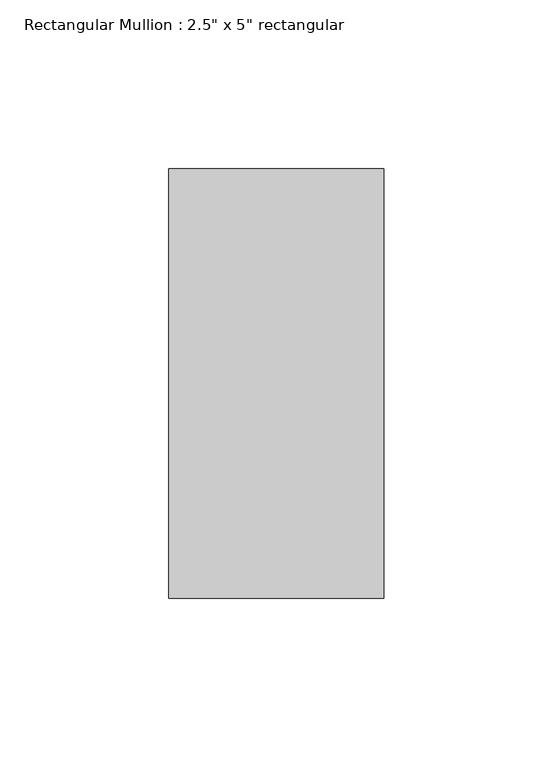
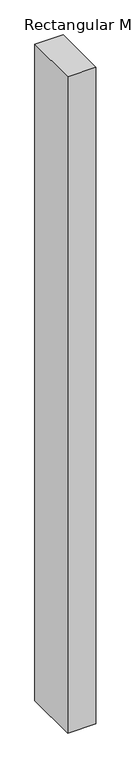
"""IFC4 building model written with IfcOpenShell, lengths in millimetres: member geometry."""

from ifc_helpers import new_model, si_unit, frame, origin, place, context, project, spatial, polyline, outline, extrude, source, transform, mapped, element, save


def member_22561c7a(model_context):
    return source(origin(), model_context, "Body", "SweptSolid", [
        extrude(outline(polyline([(0.0, 63.5), (0.0, -63.5), (-63.5, -63.5), (-63.5, 63.5), (0.0, 63.5)])), frame((0.0, 0.0, -1557.4533749), z_axis=(0.0, 0.0, 1.0), x_axis=(1.0, 0.0, 0.0)), (0.0, 0.0, 1.0), 1557.4533749),
    ])


if __name__ == "__main__":
    model = new_model("IFC4")
    model_context = context("Model", 3, world=origin())
    ifc_project = project(units=[si_unit("LENGTHUNIT", "METRE", prefix="MILLI")], contexts=[model_context])
    site = spatial("IfcSite", under=ifc_project)
    building = spatial("IfcBuilding", under=site)
    placement = place(None, origin())
    member_shape = member_22561c7a(model_context)
    element("IfcMember", 1, ObjectType="Rectangular Mullion : 2.5\" x 5\" rectangular", at=placement, inside=building, context=model_context, shape_type="MappedRepresentation", body=[
        mapped(member_shape, transform((0.0, 0.0, 0.0), x_axis=(1.0, 0.0, 0.0), y_axis=(0.0, 1.0, 0.0), z_axis=(0.0, 0.0, 1.0))),
    ])
    save(model, "model.ifc")

# Revit data of these elements
# Type "Rectangular Mullion : 2.5\" x 5\" rectangular"
#   built-in parameter 1007304 = 0.416667 (stored number, unit not read)
#   built-in parameter 1007301 = 0.104167 (stored number, unit not read)
#   built-in parameter 1007300 = 0.104167 (stored number, unit not read)
# Element 1 (IfcMember, "Rectangular Mullion : 2.5\" x 5\" rectangular")
#   Materials on its faces: "Aluminum"
# Materials
#   "Aluminum": class "Metal", colour RGB 247 247 247, transparency 0, Description = "Aluminum 6061", Cost = 0
